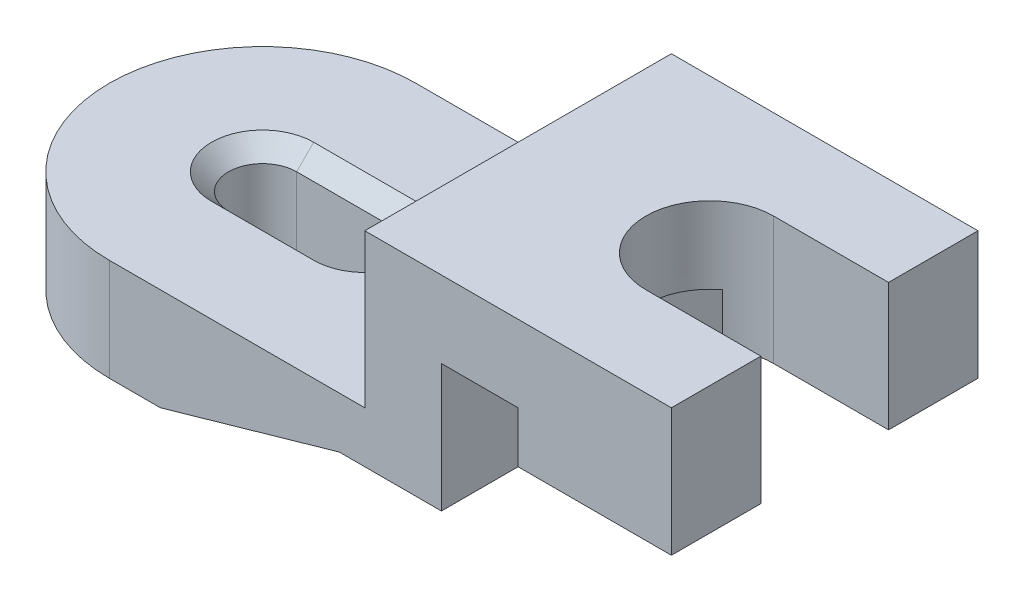
ISO-10303-21;
HEADER;
FILE_DESCRIPTION(('STEP AP214'),'2;1');
FILE_NAME('part.step','',(''),(''),'','','');
FILE_SCHEMA(('AUTOMOTIVE_DESIGN { 1 0 10303 214 1 1 1 1 }'));
ENDSEC;
DATA;
#1=APPLICATION_CONTEXT('core data for automotive mechanical design processes');
#2=APPLICATION_PROTOCOL_DEFINITION('international standard','automotive_design',2000,#1);
#3=PRODUCT_CONTEXT('',#1,'mechanical');
#4=PRODUCT('Part','Part','',(#3));
#5=PRODUCT_RELATED_PRODUCT_CATEGORY('part','',(#4));
#6=PRODUCT_DEFINITION_FORMATION('','',#4);
#7=PRODUCT_DEFINITION_CONTEXT('part definition',#1,'design');
#8=PRODUCT_DEFINITION('design','',#6,#7);
#9=PRODUCT_DEFINITION_SHAPE('','',#8);
#10=(LENGTH_UNIT() NAMED_UNIT(*) SI_UNIT(.MILLI.,.METRE.));
#11=(NAMED_UNIT(*) PLANE_ANGLE_UNIT() SI_UNIT($,.RADIAN.));
#12=(NAMED_UNIT(*) SI_UNIT($,.STERADIAN.) SOLID_ANGLE_UNIT());
#13=UNCERTAINTY_MEASURE_WITH_UNIT(LENGTH_MEASURE(1.E-05),#10,'distance_accuracy_value','');
#14=(GEOMETRIC_REPRESENTATION_CONTEXT(3) GLOBAL_UNCERTAINTY_ASSIGNED_CONTEXT((#13)) GLOBAL_UNIT_ASSIGNED_CONTEXT((#10,
#11,#12)) REPRESENTATION_CONTEXT('',''));
#15=CARTESIAN_POINT('',(0.,0.,0.));
#16=DIRECTION('',(0.,0.,1.));
#17=DIRECTION('',(1.,0.,0.));
#18=AXIS2_PLACEMENT_3D('',#15,#16,#17);
#19=CARTESIAN_POINT('',(0.,0.,0.));
#20=DIRECTION('',(0.,1.,0.));
#21=DIRECTION('',(0.,0.,1.));
#22=AXIS2_PLACEMENT_3D('',#19,#20,#21);
#23=PLANE('',#22);
#24=DIRECTION('',(0.,0.,-1.));
#25=VECTOR('',#24,1.);
#26=CARTESIAN_POINT('',(6.00000000000001,0.,208.));
#27=LINE('',#26,#25);
#28=CARTESIAN_POINT('',(6.00000000000001,0.,18.));
#29=VERTEX_POINT('',#28);
#30=CARTESIAN_POINT('',(6.00000000000001,0.,4.));
#31=VERTEX_POINT('',#30);
#32=EDGE_CURVE('E214',#29,#31,#27,.T.);
#33=ORIENTED_EDGE('',*,*,#32,.F.);
#34=DIRECTION('',(1.,0.,0.));
#35=VECTOR('',#34,1.);
#36=CARTESIAN_POINT('',(0.,0.,18.));
#37=LINE('',#36,#35);
#38=CARTESIAN_POINT('',(0.,0.,18.));
#39=VERTEX_POINT('',#38);
#40=EDGE_CURVE('E222',#39,#29,#37,.T.);
#41=ORIENTED_EDGE('',*,*,#40,.F.);
#42=CARTESIAN_POINT('',(0.,0.,0.));
#43=DIRECTION('',(0.,1.,0.));
#44=DIRECTION('',(0.,0.,1.));
#45=AXIS2_PLACEMENT_3D('',#42,#43,#44);
#46=CIRCLE('',#45,18.);
#47=CARTESIAN_POINT('',(0.,0.,-18.));
#48=VERTEX_POINT('',#47);
#49=EDGE_CURVE('E254',#48,#39,#46,.T.);
#50=ORIENTED_EDGE('',*,*,#49,.F.);
#51=DIRECTION('',(1.,0.,0.));
#52=VECTOR('',#51,1.);
#53=CARTESIAN_POINT('',(0.,0.,-18.));
#54=LINE('',#53,#52);
#55=CARTESIAN_POINT('',(6.00000000000001,0.,-18.));
#56=VERTEX_POINT('',#55);
#57=EDGE_CURVE('E234',#48,#56,#54,.T.);
#58=ORIENTED_EDGE('',*,*,#57,.T.);
#59=CARTESIAN_POINT('',(6.00000000000001,0.,-4.));
#60=VERTEX_POINT('',#59);
#61=EDGE_CURVE('E226',#60,#56,#27,.T.);
#62=ORIENTED_EDGE('',*,*,#61,.F.);
#63=DIRECTION('',(-1.,0.,0.));
#64=VECTOR('',#63,1.);
#65=CARTESIAN_POINT('',(0.,0.,-3.99999999999999));
#66=LINE('',#65,#64);
#67=CARTESIAN_POINT('',(0.,0.,-3.99999999999999));
#68=VERTEX_POINT('',#67);
#69=EDGE_CURVE('E259',#60,#68,#66,.T.);
#70=ORIENTED_EDGE('',*,*,#69,.T.);
#71=CARTESIAN_POINT('',(0.,0.,0.));
#72=DIRECTION('',(0.,1.,0.));
#73=DIRECTION('',(0.,0.,1.));
#74=AXIS2_PLACEMENT_3D('',#71,#72,#73);
#75=CIRCLE('',#74,3.99999999999999);
#76=CARTESIAN_POINT('',(0.,0.,3.99999999999999));
#77=VERTEX_POINT('',#76);
#78=EDGE_CURVE('E262',#68,#77,#75,.T.);
#79=ORIENTED_EDGE('',*,*,#78,.T.);
#80=DIRECTION('',(1.,0.,0.));
#81=VECTOR('',#80,1.);
#82=CARTESIAN_POINT('',(0.,0.,3.99999999999999));
#83=LINE('',#82,#81);
#84=EDGE_CURVE('E227',#77,#31,#83,.T.);
#85=ORIENTED_EDGE('',*,*,#84,.T.);
#86=EDGE_LOOP('',(#33,#41,#50,#58,#62,#70,#79,#85));
#87=FACE_BOUND('',#86,.T.);
#88=ADVANCED_FACE('F43',(#87),#23,.F.);
#89=CARTESIAN_POINT('',(0.,0.,-18.));
#90=DIRECTION('',(0.,0.,1.));
#91=DIRECTION('',(1.,0.,0.));
#92=AXIS2_PLACEMENT_3D('',#89,#90,#91);
#93=PLANE('',#92);
#94=DIRECTION('',(1.,0.,0.));
#95=VECTOR('',#94,1.);
#96=CARTESIAN_POINT('',(0.,5.99999999999999,-18.));
#97=LINE('',#96,#95);
#98=CARTESIAN_POINT('',(27.,6.,-18.));
#99=VERTEX_POINT('',#98);
#100=CARTESIAN_POINT('',(39.,6.,-18.));
#101=VERTEX_POINT('',#100);
#102=EDGE_CURVE('E59',#99,#101,#97,.T.);
#103=ORIENTED_EDGE('',*,*,#102,.F.);
#104=DIRECTION('',(0.961523947640823,0.274721127897378,0.));
#105=VECTOR('',#104,1.);
#106=CARTESIAN_POINT('',(0.452830188679243,-1.58490566037736,-18.));
#107=LINE('',#106,#105);
#108=EDGE_CURVE('E219',#56,#99,#107,.T.);
#109=ORIENTED_EDGE('',*,*,#108,.F.);
#110=ORIENTED_EDGE('',*,*,#57,.F.);
#111=DIRECTION('',(0.,1.,0.));
#112=VECTOR('',#111,1.);
#113=CARTESIAN_POINT('',(0.,0.,-18.));
#114=LINE('',#113,#112);
#115=CARTESIAN_POINT('',(0.,12.,-18.));
#116=VERTEX_POINT('',#115);
#117=EDGE_CURVE('E249',#48,#116,#114,.T.);
#118=ORIENTED_EDGE('',*,*,#117,.T.);
#119=DIRECTION('',(1.,0.,0.));
#120=VECTOR('',#119,1.);
#121=CARTESIAN_POINT('',(0.,12.,-18.));
#122=LINE('',#121,#120);
#123=CARTESIAN_POINT('',(30.,12.,-18.));
#124=VERTEX_POINT('',#123);
#125=EDGE_CURVE('E232',#116,#124,#122,.T.);
#126=ORIENTED_EDGE('',*,*,#125,.T.);
#127=DIRECTION('',(0.,-1.,0.));
#128=VECTOR('',#127,1.);
#129=CARTESIAN_POINT('',(30.,12.,-18.));
#130=LINE('',#129,#128);
#131=CARTESIAN_POINT('',(30.,30.,-18.));
#132=VERTEX_POINT('',#131);
#133=EDGE_CURVE('E330',#132,#124,#130,.T.);
#134=ORIENTED_EDGE('',*,*,#133,.F.);
#135=DIRECTION('',(-1.,0.,0.));
#136=VECTOR('',#135,1.);
#137=CARTESIAN_POINT('',(30.,30.,-18.));
#138=LINE('',#137,#136);
#139=CARTESIAN_POINT('',(66.,30.,-18.));
#140=VERTEX_POINT('',#139);
#141=EDGE_CURVE('E335',#140,#132,#138,.T.);
#142=ORIENTED_EDGE('',*,*,#141,.F.);
#143=DIRECTION('',(0.,1.,0.));
#144=VECTOR('',#143,1.);
#145=CARTESIAN_POINT('',(66.,0.,-18.));
#146=LINE('',#145,#144);
#147=CARTESIAN_POINT('',(66.,15.,-18.));
#148=VERTEX_POINT('',#147);
#149=EDGE_CURVE('E326',#148,#140,#146,.T.);
#150=ORIENTED_EDGE('',*,*,#149,.F.);
#151=DIRECTION('',(-1.,0.,0.));
#152=VECTOR('',#151,1.);
#153=CARTESIAN_POINT('',(0.,15.,-18.));
#154=LINE('',#153,#152);
#155=CARTESIAN_POINT('',(48.,15.,-18.));
#156=VERTEX_POINT('',#155);
#157=EDGE_CURVE('E432',#148,#156,#154,.T.);
#158=ORIENTED_EDGE('',*,*,#157,.T.);
#159=DIRECTION('',(0.,-1.,0.));
#160=VECTOR('',#159,1.);
#161=CARTESIAN_POINT('',(48.,0.,-18.));
#162=LINE('',#161,#160);
#163=CARTESIAN_POINT('',(48.,21.,-18.));
#164=VERTEX_POINT('',#163);
#165=EDGE_CURVE('E297',#164,#156,#162,.T.);
#166=ORIENTED_EDGE('',*,*,#165,.F.);
#167=DIRECTION('',(-1.,0.,0.));
#168=VECTOR('',#167,1.);
#169=CARTESIAN_POINT('',(0.,21.,-18.));
#170=LINE('',#169,#168);
#171=CARTESIAN_POINT('',(39.,21.,-18.));
#172=VERTEX_POINT('',#171);
#173=EDGE_CURVE('E311',#164,#172,#170,.T.);
#174=ORIENTED_EDGE('',*,*,#173,.T.);
#175=DIRECTION('',(0.,-1.,0.));
#176=VECTOR('',#175,1.);
#177=CARTESIAN_POINT('',(39.,0.,-18.));
#178=LINE('',#177,#176);
#179=EDGE_CURVE('E291',#172,#101,#178,.T.);
#180=ORIENTED_EDGE('',*,*,#179,.T.);
#181=EDGE_LOOP('',(#103,#109,#110,#118,#126,#134,#142,#150,#158,#166,#174,#180));
#182=FACE_BOUND('',#181,.T.);
#183=ADVANCED_FACE('F443',(#182),#93,.F.);
#184=CARTESIAN_POINT('',(0.,0.,18.));
#185=DIRECTION('',(0.,0.,1.));
#186=DIRECTION('',(1.,0.,0.));
#187=AXIS2_PLACEMENT_3D('',#184,#185,#186);
#188=PLANE('',#187);
#189=DIRECTION('',(0.961523947640823,0.274721127897378,0.));
#190=VECTOR('',#189,1.);
#191=CARTESIAN_POINT('',(0.452830188679243,-1.58490566037736,18.));
#192=LINE('',#191,#190);
#193=CARTESIAN_POINT('',(27.,6.,18.));
#194=VERTEX_POINT('',#193);
#195=EDGE_CURVE('E208',#29,#194,#192,.T.);
#196=ORIENTED_EDGE('',*,*,#195,.T.);
#197=DIRECTION('',(1.,0.,0.));
#198=VECTOR('',#197,1.);
#199=CARTESIAN_POINT('',(0.,5.99999999999999,18.));
#200=LINE('',#199,#198);
#201=CARTESIAN_POINT('',(39.,6.,18.));
#202=VERTEX_POINT('',#201);
#203=EDGE_CURVE('E283',#194,#202,#200,.T.);
#204=ORIENTED_EDGE('',*,*,#203,.T.);
#205=DIRECTION('',(0.,-1.,0.));
#206=VECTOR('',#205,1.);
#207=CARTESIAN_POINT('',(39.,0.,18.));
#208=LINE('',#207,#206);
#209=CARTESIAN_POINT('',(39.,21.,18.));
#210=VERTEX_POINT('',#209);
#211=EDGE_CURVE('E279',#210,#202,#208,.T.);
#212=ORIENTED_EDGE('',*,*,#211,.F.);
#213=DIRECTION('',(-1.,0.,0.));
#214=VECTOR('',#213,1.);
#215=CARTESIAN_POINT('',(0.,21.,18.));
#216=LINE('',#215,#214);
#217=CARTESIAN_POINT('',(48.,21.,18.));
#218=VERTEX_POINT('',#217);
#219=EDGE_CURVE('E307',#218,#210,#216,.T.);
#220=ORIENTED_EDGE('',*,*,#219,.F.);
#221=DIRECTION('',(0.,-1.,0.));
#222=VECTOR('',#221,1.);
#223=CARTESIAN_POINT('',(48.,0.,18.));
#224=LINE('',#223,#222);
#225=CARTESIAN_POINT('',(48.,15.,18.));
#226=VERTEX_POINT('',#225);
#227=EDGE_CURVE('E298',#218,#226,#224,.T.);
#228=ORIENTED_EDGE('',*,*,#227,.T.);
#229=DIRECTION('',(-1.,0.,0.));
#230=VECTOR('',#229,1.);
#231=CARTESIAN_POINT('',(0.,15.,18.));
#232=LINE('',#231,#230);
#233=CARTESIAN_POINT('',(66.,15.,18.));
#234=VERTEX_POINT('',#233);
#235=EDGE_CURVE('E433',#234,#226,#232,.T.);
#236=ORIENTED_EDGE('',*,*,#235,.F.);
#237=DIRECTION('',(0.,1.,0.));
#238=VECTOR('',#237,1.);
#239=CARTESIAN_POINT('',(66.,30.,18.));
#240=LINE('',#239,#238);
#241=CARTESIAN_POINT('',(66.,30.,18.));
#242=VERTEX_POINT('',#241);
#243=EDGE_CURVE('E323',#234,#242,#240,.T.);
#244=ORIENTED_EDGE('',*,*,#243,.T.);
#245=DIRECTION('',(-1.,0.,0.));
#246=VECTOR('',#245,1.);
#247=CARTESIAN_POINT('',(30.,30.,18.));
#248=LINE('',#247,#246);
#249=CARTESIAN_POINT('',(30.,30.,18.));
#250=VERTEX_POINT('',#249);
#251=EDGE_CURVE('E336',#242,#250,#248,.T.);
#252=ORIENTED_EDGE('',*,*,#251,.T.);
#253=DIRECTION('',(0.,-1.,0.));
#254=VECTOR('',#253,1.);
#255=CARTESIAN_POINT('',(30.,12.,18.));
#256=LINE('',#255,#254);
#257=CARTESIAN_POINT('',(30.,12.,18.));
#258=VERTEX_POINT('',#257);
#259=EDGE_CURVE('E334',#250,#258,#256,.T.);
#260=ORIENTED_EDGE('',*,*,#259,.T.);
#261=DIRECTION('',(1.,0.,0.));
#262=VECTOR('',#261,1.);
#263=CARTESIAN_POINT('',(0.,12.,18.));
#264=LINE('',#263,#262);
#265=CARTESIAN_POINT('',(0.,12.,18.));
#266=VERTEX_POINT('',#265);
#267=EDGE_CURVE('E244',#266,#258,#264,.T.);
#268=ORIENTED_EDGE('',*,*,#267,.F.);
#269=DIRECTION('',(0.,1.,0.));
#270=VECTOR('',#269,1.);
#271=CARTESIAN_POINT('',(0.,0.,18.));
#272=LINE('',#271,#270);
#273=EDGE_CURVE('E231',#39,#266,#272,.T.);
#274=ORIENTED_EDGE('',*,*,#273,.F.);
#275=ORIENTED_EDGE('',*,*,#40,.T.);
#276=EDGE_LOOP('',(#196,#204,#212,#220,#228,#236,#244,#252,#260,#268,#274,#275));
#277=FACE_BOUND('',#276,.T.);
#278=ADVANCED_FACE('F233',(#277),#188,.T.);
#279=CARTESIAN_POINT('',(0.,-8.,3.99999999999999));
#280=DIRECTION('',(0.,0.,1.));
#281=DIRECTION('',(1.,0.,0.));
#282=AXIS2_PLACEMENT_3D('',#279,#280,#281);
#283=PLANE('',#282);
#284=DIRECTION('',(0.961523947640823,0.274721127897378,0.));
#285=VECTOR('',#284,1.);
#286=CARTESIAN_POINT('',(-1.66037735849057,-2.18867924528302,3.99999999999999));
#287=LINE('',#286,#285);
#288=CARTESIAN_POINT('',(12.,1.71428571428571,3.99999999999999));
#289=VERTEX_POINT('',#288);
#290=EDGE_CURVE('E216',#31,#289,#287,.T.);
#291=ORIENTED_EDGE('',*,*,#290,.F.);
#292=ORIENTED_EDGE('',*,*,#84,.F.);
#293=DIRECTION('',(0.,1.,0.));
#294=VECTOR('',#293,1.);
#295=CARTESIAN_POINT('',(0.,-8.,3.99999999999999));
#296=LINE('',#295,#294);
#297=CARTESIAN_POINT('',(0.,10.,3.99999999999999));
#298=VERTEX_POINT('',#297);
#299=EDGE_CURVE('E349',#77,#298,#296,.T.);
#300=ORIENTED_EDGE('',*,*,#299,.T.);
#301=DIRECTION('',(1.,0.,0.));
#302=VECTOR('',#301,1.);
#303=CARTESIAN_POINT('',(0.,10.,3.99999999999999));
#304=LINE('',#303,#302);
#305=CARTESIAN_POINT('',(12.,10.,3.99999999999999));
#306=VERTEX_POINT('',#305);
#307=EDGE_CURVE('E245',#298,#306,#304,.T.);
#308=ORIENTED_EDGE('',*,*,#307,.T.);
#309=DIRECTION('',(0.,1.,0.));
#310=VECTOR('',#309,1.);
#311=CARTESIAN_POINT('',(12.,-8.,3.99999999999999));
#312=LINE('',#311,#310);
#313=EDGE_CURVE('E343',#289,#306,#312,.T.);
#314=ORIENTED_EDGE('',*,*,#313,.F.);
#315=EDGE_LOOP('',(#291,#292,#300,#308,#314));
#316=FACE_BOUND('',#315,.T.);
#317=ADVANCED_FACE('F392',(#316),#283,.F.);
#318=CARTESIAN_POINT('',(0.,-8.,-3.99999999999999));
#319=DIRECTION('',(0.,0.,-1.));
#320=DIRECTION('',(-1.,0.,0.));
#321=AXIS2_PLACEMENT_3D('',#318,#319,#320);
#322=PLANE('',#321);
#323=DIRECTION('',(-0.961523947640823,-0.274721127897378,0.));
#324=VECTOR('',#323,1.);
#325=CARTESIAN_POINT('',(-1.66037735849057,-2.18867924528302,-3.99999999999999));
#326=LINE('',#325,#324);
#327=CARTESIAN_POINT('',(12.,1.71428571428571,-3.99999999999999));
#328=VERTEX_POINT('',#327);
#329=EDGE_CURVE('E408',#328,#60,#326,.T.);
#330=ORIENTED_EDGE('',*,*,#329,.F.);
#331=DIRECTION('',(0.,1.,0.));
#332=VECTOR('',#331,1.);
#333=CARTESIAN_POINT('',(12.,-8.,-3.99999999999999));
#334=LINE('',#333,#332);
#335=CARTESIAN_POINT('',(12.,10.,-3.99999999999999));
#336=VERTEX_POINT('',#335);
#337=EDGE_CURVE('E353',#328,#336,#334,.T.);
#338=ORIENTED_EDGE('',*,*,#337,.T.);
#339=DIRECTION('',(-1.,0.,0.));
#340=VECTOR('',#339,1.);
#341=CARTESIAN_POINT('',(0.,10.,-3.99999999999999));
#342=LINE('',#341,#340);
#343=CARTESIAN_POINT('',(0.,10.,-3.99999999999999));
#344=VERTEX_POINT('',#343);
#345=EDGE_CURVE('E372',#336,#344,#342,.T.);
#346=ORIENTED_EDGE('',*,*,#345,.T.);
#347=DIRECTION('',(0.,1.,0.));
#348=VECTOR('',#347,1.);
#349=CARTESIAN_POINT('',(0.,-8.,-3.99999999999999));
#350=LINE('',#349,#348);
#351=EDGE_CURVE('E351',#68,#344,#350,.T.);
#352=ORIENTED_EDGE('',*,*,#351,.F.);
#353=ORIENTED_EDGE('',*,*,#69,.F.);
#354=EDGE_LOOP('',(#330,#338,#346,#352,#353));
#355=FACE_BOUND('',#354,.T.);
#356=ADVANCED_FACE('F409',(#355),#322,.F.);
#357=CARTESIAN_POINT('',(12.,-8.,0.));
#358=DIRECTION('',(0.,1.,0.));
#359=DIRECTION('',(0.,0.,1.));
#360=AXIS2_PLACEMENT_3D('',#357,#358,#359);
#361=CYLINDRICAL_SURFACE('',#360,3.99999999999999);
#362=CARTESIAN_POINT('',(12.,1.71428571428571,0.));
#363=DIRECTION('',(0.274721127897378,-0.961523947640823,0.));
#364=DIRECTION('',(0.961523947640823,0.274721127897378,0.));
#365=AXIS2_PLACEMENT_3D('',#362,#363,#364);
#366=ELLIPSE('',#365,4.16006279387457,3.99999999999999);
#367=EDGE_CURVE('E11',#289,#328,#366,.F.);
#368=ORIENTED_EDGE('',*,*,#367,.F.);
#369=ORIENTED_EDGE('',*,*,#313,.T.);
#370=CARTESIAN_POINT('',(12.,10.,0.));
#371=DIRECTION('',(0.,1.,0.));
#372=DIRECTION('',(0.,0.,1.));
#373=AXIS2_PLACEMENT_3D('',#370,#371,#372);
#374=CIRCLE('',#373,3.99999999999999);
#375=EDGE_CURVE('E379',#306,#336,#374,.T.);
#376=ORIENTED_EDGE('',*,*,#375,.T.);
#377=ORIENTED_EDGE('',*,*,#337,.F.);
#378=EDGE_LOOP('',(#368,#369,#376,#377));
#379=FACE_BOUND('',#378,.T.);
#380=ADVANCED_FACE('F415',(#379),#361,.F.);
#381=CARTESIAN_POINT('',(39.,0.,78.));
#382=DIRECTION('',(-1.,0.,0.));
#383=DIRECTION('',(0.,0.,1.));
#384=AXIS2_PLACEMENT_3D('',#381,#382,#383);
#385=PLANE('',#384);
#386=DIRECTION('',(0.,0.,1.));
#387=VECTOR('',#386,1.);
#388=CARTESIAN_POINT('',(39.,6.,78.));
#389=LINE('',#388,#387);
#390=EDGE_CURVE('E51',#101,#202,#389,.T.);
#391=ORIENTED_EDGE('',*,*,#390,.F.);
#392=ORIENTED_EDGE('',*,*,#179,.F.);
#393=DIRECTION('',(0.,0.,-1.));
#394=VECTOR('',#393,1.);
#395=CARTESIAN_POINT('',(39.,21.,78.));
#396=LINE('',#395,#394);
#397=EDGE_CURVE('E292',#210,#172,#396,.T.);
#398=ORIENTED_EDGE('',*,*,#397,.F.);
#399=ORIENTED_EDGE('',*,*,#211,.T.);
#400=EDGE_LOOP('',(#391,#392,#398,#399));
#401=FACE_BOUND('',#400,.T.);
#402=ADVANCED_FACE('F287',(#401),#385,.F.);
#403=CARTESIAN_POINT('',(52.5,-60.,0.));
#404=DIRECTION('',(0.,1.,0.));
#405=DIRECTION('',(0.,0.,1.));
#406=AXIS2_PLACEMENT_3D('',#403,#404,#405);
#407=CYLINDRICAL_SURFACE('',#406,7.5);
#408=DIRECTION('',(0.,1.,0.));
#409=VECTOR('',#408,1.);
#410=CARTESIAN_POINT('',(52.5,-60.,7.5));
#411=LINE('',#410,#409);
#412=CARTESIAN_POINT('',(52.5,15.,7.5));
#413=VERTEX_POINT('',#412);
#414=CARTESIAN_POINT('',(52.5,30.,7.5));
#415=VERTEX_POINT('',#414);
#416=EDGE_CURVE('E325',#413,#415,#411,.T.);
#417=ORIENTED_EDGE('',*,*,#416,.F.);
#418=CARTESIAN_POINT('',(52.5,15.,0.));
#419=DIRECTION('',(0.,1.,0.));
#420=DIRECTION('',(0.,0.,1.));
#421=AXIS2_PLACEMENT_3D('',#418,#419,#420);
#422=CIRCLE('',#421,7.5);
#423=CARTESIAN_POINT('',(48.,15.,5.99999999999999));
#424=VERTEX_POINT('',#423);
#425=EDGE_CURVE('E426',#413,#424,#422,.F.);
#426=ORIENTED_EDGE('',*,*,#425,.T.);
#427=DIRECTION('',(0.,1.,0.));
#428=VECTOR('',#427,1.);
#429=CARTESIAN_POINT('',(48.,-60.,5.99999999999999));
#430=LINE('',#429,#428);
#431=CARTESIAN_POINT('',(48.,21.,5.99999999999999));
#432=VERTEX_POINT('',#431);
#433=EDGE_CURVE('E273',#432,#424,#430,.F.);
#434=ORIENTED_EDGE('',*,*,#433,.F.);
#435=CARTESIAN_POINT('',(52.5,21.,0.));
#436=DIRECTION('',(0.,1.,0.));
#437=DIRECTION('',(0.,0.,1.));
#438=AXIS2_PLACEMENT_3D('',#435,#436,#437);
#439=CIRCLE('',#438,7.5);
#440=CARTESIAN_POINT('',(48.,21.,-6.00000000000001));
#441=VERTEX_POINT('',#440);
#442=EDGE_CURVE('E275',#432,#441,#439,.F.);
#443=ORIENTED_EDGE('',*,*,#442,.T.);
#444=DIRECTION('',(0.,1.,0.));
#445=VECTOR('',#444,1.);
#446=CARTESIAN_POINT('',(48.,-60.,-6.));
#447=LINE('',#446,#445);
#448=CARTESIAN_POINT('',(48.,15.,-6.));
#449=VERTEX_POINT('',#448);
#450=EDGE_CURVE('E267',#449,#441,#447,.T.);
#451=ORIENTED_EDGE('',*,*,#450,.F.);
#452=CARTESIAN_POINT('',(52.5,15.,-7.5));
#453=VERTEX_POINT('',#452);
#454=EDGE_CURVE('E67',#449,#453,#422,.F.);
#455=ORIENTED_EDGE('',*,*,#454,.T.);
#456=DIRECTION('',(0.,1.,0.));
#457=VECTOR('',#456,1.);
#458=CARTESIAN_POINT('',(52.5,-60.,-7.5));
#459=LINE('',#458,#457);
#460=CARTESIAN_POINT('',(52.5,30.,-7.5));
#461=VERTEX_POINT('',#460);
#462=EDGE_CURVE('E324',#453,#461,#459,.T.);
#463=ORIENTED_EDGE('',*,*,#462,.T.);
#464=CARTESIAN_POINT('',(52.5,30.,0.));
#465=DIRECTION('',(0.,1.,0.));
#466=DIRECTION('',(0.,0.,1.));
#467=AXIS2_PLACEMENT_3D('',#464,#465,#466);
#468=CIRCLE('',#467,7.5);
#469=EDGE_CURVE('E313',#461,#415,#468,.T.);
#470=ORIENTED_EDGE('',*,*,#469,.T.);
#471=EDGE_LOOP('',(#417,#426,#434,#443,#451,#455,#463,#470));
#472=FACE_BOUND('',#471,.T.);
#473=ADVANCED_FACE('F503',(#472),#407,.F.);
#474=CARTESIAN_POINT('',(30.,30.,-18.));
#475=DIRECTION('',(0.,1.,0.));
#476=DIRECTION('',(0.,0.,1.));
#477=AXIS2_PLACEMENT_3D('',#474,#475,#476);
#478=PLANE('',#477);
#479=ORIENTED_EDGE('',*,*,#469,.F.);
#480=DIRECTION('',(1.,0.,0.));
#481=VECTOR('',#480,1.);
#482=CARTESIAN_POINT('',(0.,30.,-7.5));
#483=LINE('',#482,#481);
#484=CARTESIAN_POINT('',(66.,30.,-7.5));
#485=VERTEX_POINT('',#484);
#486=EDGE_CURVE('E316',#461,#485,#483,.T.);
#487=ORIENTED_EDGE('',*,*,#486,.T.);
#488=DIRECTION('',(0.,0.,1.));
#489=VECTOR('',#488,1.);
#490=CARTESIAN_POINT('',(66.,30.,-18.));
#491=LINE('',#490,#489);
#492=EDGE_CURVE('E347',#140,#485,#491,.T.);
#493=ORIENTED_EDGE('',*,*,#492,.F.);
#494=ORIENTED_EDGE('',*,*,#141,.T.);
#495=DIRECTION('',(0.,0.,1.));
#496=VECTOR('',#495,1.);
#497=CARTESIAN_POINT('',(30.,30.,-18.));
#498=LINE('',#497,#496);
#499=EDGE_CURVE('E344',#132,#250,#498,.T.);
#500=ORIENTED_EDGE('',*,*,#499,.T.);
#501=ORIENTED_EDGE('',*,*,#251,.F.);
#502=CARTESIAN_POINT('',(66.,30.,7.49999999999999));
#503=VERTEX_POINT('',#502);
#504=EDGE_CURVE('E337',#503,#242,#491,.T.);
#505=ORIENTED_EDGE('',*,*,#504,.F.);
#506=DIRECTION('',(1.,0.,0.));
#507=VECTOR('',#506,1.);
#508=CARTESIAN_POINT('',(0.,30.,7.5));
#509=LINE('',#508,#507);
#510=EDGE_CURVE('E320',#415,#503,#509,.T.);
#511=ORIENTED_EDGE('',*,*,#510,.F.);
#512=EDGE_LOOP('',(#479,#487,#493,#494,#500,#501,#505,#511));
#513=FACE_BOUND('',#512,.T.);
#514=ADVANCED_FACE('F501',(#513),#478,.T.);
#515=CARTESIAN_POINT('',(66.,30.,-18.));
#516=DIRECTION('',(1.,0.,0.));
#517=DIRECTION('',(0.,0.,-1.));
#518=AXIS2_PLACEMENT_3D('',#515,#516,#517);
#519=PLANE('',#518);
#520=DIRECTION('',(0.,0.,-1.));
#521=VECTOR('',#520,1.);
#522=CARTESIAN_POINT('',(66.,15.,91.));
#523=LINE('',#522,#521);
#524=CARTESIAN_POINT('',(66.,15.,-7.50000000000001));
#525=VERTEX_POINT('',#524);
#526=EDGE_CURVE('E418',#525,#148,#523,.T.);
#527=ORIENTED_EDGE('',*,*,#526,.T.);
#528=ORIENTED_EDGE('',*,*,#149,.T.);
#529=ORIENTED_EDGE('',*,*,#492,.T.);
#530=DIRECTION('',(0.,-1.,0.));
#531=VECTOR('',#530,1.);
#532=CARTESIAN_POINT('',(66.,30.,-7.5));
#533=LINE('',#532,#531);
#534=EDGE_CURVE('E266',#485,#525,#533,.T.);
#535=ORIENTED_EDGE('',*,*,#534,.T.);
#536=EDGE_LOOP('',(#527,#528,#529,#535));
#537=FACE_BOUND('',#536,.T.);
#538=ADVANCED_FACE('F499',(#537),#519,.T.);
#539=CARTESIAN_POINT('',(0.,12.,0.));
#540=DIRECTION('',(0.,-1.,0.));
#541=DIRECTION('',(0.,0.,-1.));
#542=AXIS2_PLACEMENT_3D('',#539,#540,#541);
#543=CYLINDRICAL_SURFACE('',#542,18.);
#544=CARTESIAN_POINT('',(0.,12.,0.));
#545=DIRECTION('',(0.,1.,0.));
#546=DIRECTION('',(0.,0.,1.));
#547=AXIS2_PLACEMENT_3D('',#544,#545,#546);
#548=CIRCLE('',#547,18.);
#549=EDGE_CURVE('E253',#116,#266,#548,.T.);
#550=ORIENTED_EDGE('',*,*,#549,.F.);
#551=ORIENTED_EDGE('',*,*,#117,.F.);
#552=ORIENTED_EDGE('',*,*,#49,.T.);
#553=ORIENTED_EDGE('',*,*,#273,.T.);
#554=EDGE_LOOP('',(#550,#551,#552,#553));
#555=FACE_BOUND('',#554,.T.);
#556=ADVANCED_FACE('F44',(#555),#543,.T.);
#557=CARTESIAN_POINT('',(0.,12.,0.));
#558=DIRECTION('',(0.,1.,0.));
#559=DIRECTION('',(0.,0.,1.));
#560=AXIS2_PLACEMENT_3D('',#557,#558,#559);
#561=PLANE('',#560);
#562=CARTESIAN_POINT('',(0.,12.,0.));
#563=DIRECTION('',(0.,1.,0.));
#564=DIRECTION('',(0.,0.,1.));
#565=AXIS2_PLACEMENT_3D('',#562,#563,#564);
#566=CIRCLE('',#565,6.);
#567=CARTESIAN_POINT('',(0.,12.,-6.));
#568=VERTEX_POINT('',#567);
#569=CARTESIAN_POINT('',(0.,12.,6.));
#570=VERTEX_POINT('',#569);
#571=EDGE_CURVE('E354',#568,#570,#566,.T.);
#572=ORIENTED_EDGE('',*,*,#571,.F.);
#573=DIRECTION('',(-1.,0.,0.));
#574=VECTOR('',#573,1.);
#575=CARTESIAN_POINT('',(0.,12.,-6.));
#576=LINE('',#575,#574);
#577=CARTESIAN_POINT('',(12.,12.,-6.));
#578=VERTEX_POINT('',#577);
#579=EDGE_CURVE('E364',#578,#568,#576,.T.);
#580=ORIENTED_EDGE('',*,*,#579,.F.);
#581=CARTESIAN_POINT('',(12.,12.,0.));
#582=DIRECTION('',(0.,1.,0.));
#583=DIRECTION('',(0.,0.,1.));
#584=AXIS2_PLACEMENT_3D('',#581,#582,#583);
#585=CIRCLE('',#584,6.);
#586=CARTESIAN_POINT('',(12.,12.,6.));
#587=VERTEX_POINT('',#586);
#588=EDGE_CURVE('E363',#587,#578,#585,.T.);
#589=ORIENTED_EDGE('',*,*,#588,.F.);
#590=DIRECTION('',(1.,0.,0.));
#591=VECTOR('',#590,1.);
#592=CARTESIAN_POINT('',(0.,12.,6.));
#593=LINE('',#592,#591);
#594=EDGE_CURVE('E356',#570,#587,#593,.T.);
#595=ORIENTED_EDGE('',*,*,#594,.F.);
#596=EDGE_LOOP('',(#572,#580,#589,#595));
#597=FACE_BOUND('',#596,.T.);
#598=ORIENTED_EDGE('',*,*,#549,.T.);
#599=ORIENTED_EDGE('',*,*,#267,.T.);
#600=DIRECTION('',(0.,0.,1.));
#601=VECTOR('',#600,1.);
#602=CARTESIAN_POINT('',(30.,12.,0.));
#603=LINE('',#602,#601);
#604=EDGE_CURVE('E237',#124,#258,#603,.T.);
#605=ORIENTED_EDGE('',*,*,#604,.F.);
#606=ORIENTED_EDGE('',*,*,#125,.F.);
#607=EDGE_LOOP('',(#598,#599,#605,#606));
#608=FACE_BOUND('',#607,.T.);
#609=ADVANCED_FACE('F469',(#597,#608),#561,.T.);
#610=CARTESIAN_POINT('',(0.,12.,0.));
#611=DIRECTION('',(0.,1.,0.));
#612=DIRECTION('',(0.,0.,1.));
#613=AXIS2_PLACEMENT_3D('',#610,#611,#612);
#614=CONICAL_SURFACE('',#613,6.,0.78539816339745);
#615=ORIENTED_EDGE('',*,*,#571,.T.);
#616=DIRECTION('',(0.,0.707106781186546,0.707106781186549));
#617=VECTOR('',#616,1.);
#618=CARTESIAN_POINT('',(0.,12.,6.));
#619=LINE('',#618,#617);
#620=EDGE_CURVE('E369',#298,#570,#619,.T.);
#621=ORIENTED_EDGE('',*,*,#620,.F.);
#622=CARTESIAN_POINT('',(0.,10.,0.));
#623=DIRECTION('',(0.,1.,0.));
#624=DIRECTION('',(0.,0.,1.));
#625=AXIS2_PLACEMENT_3D('',#622,#623,#624);
#626=CIRCLE('',#625,3.99999999999999);
#627=EDGE_CURVE('E370',#344,#298,#626,.T.);
#628=ORIENTED_EDGE('',*,*,#627,.F.);
#629=DIRECTION('',(0.,0.707106781186546,-0.707106781186549));
#630=VECTOR('',#629,1.);
#631=CARTESIAN_POINT('',(0.,12.,-6.));
#632=LINE('',#631,#630);
#633=EDGE_CURVE('E250',#344,#568,#632,.T.);
#634=ORIENTED_EDGE('',*,*,#633,.T.);
#635=EDGE_LOOP('',(#615,#621,#628,#634));
#636=FACE_BOUND('',#635,.T.);
#637=ADVANCED_FACE('F475',(#636),#614,.F.);
#638=CARTESIAN_POINT('',(0.,12.,-6.));
#639=DIRECTION('',(0.,-0.707106781186549,-0.707106781186546));
#640=DIRECTION('',(0.,0.707106781186546,-0.707106781186549));
#641=AXIS2_PLACEMENT_3D('',#638,#639,#640);
#642=PLANE('',#641);
#643=ORIENTED_EDGE('',*,*,#579,.T.);
#644=ORIENTED_EDGE('',*,*,#633,.F.);
#645=ORIENTED_EDGE('',*,*,#345,.F.);
#646=DIRECTION('',(0.,0.707106781186546,-0.707106781186549));
#647=VECTOR('',#646,1.);
#648=CARTESIAN_POINT('',(12.,12.,-6.));
#649=LINE('',#648,#647);
#650=EDGE_CURVE('E367',#336,#578,#649,.T.);
#651=ORIENTED_EDGE('',*,*,#650,.T.);
#652=EDGE_LOOP('',(#643,#644,#645,#651));
#653=FACE_BOUND('',#652,.T.);
#654=ADVANCED_FACE('F401',(#653),#642,.F.);
#655=CARTESIAN_POINT('',(12.,12.,0.));
#656=DIRECTION('',(0.,1.,0.));
#657=DIRECTION('',(0.,0.,1.));
#658=AXIS2_PLACEMENT_3D('',#655,#656,#657);
#659=CONICAL_SURFACE('',#658,6.,0.78539816339745);
#660=ORIENTED_EDGE('',*,*,#588,.T.);
#661=ORIENTED_EDGE('',*,*,#650,.F.);
#662=ORIENTED_EDGE('',*,*,#375,.F.);
#663=DIRECTION('',(0.,0.707106781186546,0.707106781186549));
#664=VECTOR('',#663,1.);
#665=CARTESIAN_POINT('',(12.,12.,6.));
#666=LINE('',#665,#664);
#667=EDGE_CURVE('E373',#306,#587,#666,.T.);
#668=ORIENTED_EDGE('',*,*,#667,.T.);
#669=EDGE_LOOP('',(#660,#661,#662,#668));
#670=FACE_BOUND('',#669,.T.);
#671=ADVANCED_FACE('F400',(#670),#659,.F.);
#672=CARTESIAN_POINT('',(0.,12.,6.));
#673=DIRECTION('',(0.,-0.707106781186549,0.707106781186546));
#674=DIRECTION('',(0.,-0.707106781186546,-0.707106781186549));
#675=AXIS2_PLACEMENT_3D('',#672,#673,#674);
#676=PLANE('',#675);
#677=ORIENTED_EDGE('',*,*,#594,.T.);
#678=ORIENTED_EDGE('',*,*,#667,.F.);
#679=ORIENTED_EDGE('',*,*,#307,.F.);
#680=ORIENTED_EDGE('',*,*,#620,.T.);
#681=EDGE_LOOP('',(#677,#678,#679,#680));
#682=FACE_BOUND('',#681,.T.);
#683=ADVANCED_FACE('F394',(#682),#676,.F.);
#684=CARTESIAN_POINT('',(0.,-8.,0.));
#685=DIRECTION('',(0.,1.,0.));
#686=DIRECTION('',(0.,0.,1.));
#687=AXIS2_PLACEMENT_3D('',#684,#685,#686);
#688=CYLINDRICAL_SURFACE('',#687,3.99999999999999);
#689=ORIENTED_EDGE('',*,*,#351,.T.);
#690=ORIENTED_EDGE('',*,*,#627,.T.);
#691=ORIENTED_EDGE('',*,*,#299,.F.);
#692=ORIENTED_EDGE('',*,*,#78,.F.);
#693=EDGE_LOOP('',(#689,#690,#691,#692));
#694=FACE_BOUND('',#693,.T.);
#695=ADVANCED_FACE('F481',(#694),#688,.F.);
#696=CARTESIAN_POINT('',(30.,12.,-18.));
#697=DIRECTION('',(-1.,0.,0.));
#698=DIRECTION('',(0.,0.,1.));
#699=AXIS2_PLACEMENT_3D('',#696,#697,#698);
#700=PLANE('',#699);
#701=ORIENTED_EDGE('',*,*,#133,.T.);
#702=ORIENTED_EDGE('',*,*,#604,.T.);
#703=ORIENTED_EDGE('',*,*,#259,.F.);
#704=ORIENTED_EDGE('',*,*,#499,.F.);
#705=EDGE_LOOP('',(#701,#702,#703,#704));
#706=FACE_BOUND('',#705,.T.);
#707=ADVANCED_FACE('F494',(#706),#700,.T.);
#708=CARTESIAN_POINT('',(66.,15.,7.49999999999999));
#709=VERTEX_POINT('',#708);
#710=EDGE_CURVE('E422',#234,#709,#523,.T.);
#711=ORIENTED_EDGE('',*,*,#710,.T.);
#712=DIRECTION('',(0.,-1.,0.));
#713=VECTOR('',#712,1.);
#714=CARTESIAN_POINT('',(66.,30.,7.5));
#715=LINE('',#714,#713);
#716=EDGE_CURVE('E264',#503,#709,#715,.T.);
#717=ORIENTED_EDGE('',*,*,#716,.F.);
#718=ORIENTED_EDGE('',*,*,#504,.T.);
#719=ORIENTED_EDGE('',*,*,#243,.F.);
#720=EDGE_LOOP('',(#711,#717,#718,#719));
#721=FACE_BOUND('',#720,.T.);
#722=ADVANCED_FACE('F496',(#721),#519,.T.);
#723=CARTESIAN_POINT('',(0.,-60.,-7.5));
#724=DIRECTION('',(0.,0.,1.));
#725=DIRECTION('',(1.,0.,0.));
#726=AXIS2_PLACEMENT_3D('',#723,#724,#725);
#727=PLANE('',#726);
#728=DIRECTION('',(-1.,0.,0.));
#729=VECTOR('',#728,1.);
#730=CARTESIAN_POINT('',(0.,15.,-7.5));
#731=LINE('',#730,#729);
#732=EDGE_CURVE('E431',#525,#453,#731,.T.);
#733=ORIENTED_EDGE('',*,*,#732,.F.);
#734=ORIENTED_EDGE('',*,*,#534,.F.);
#735=ORIENTED_EDGE('',*,*,#486,.F.);
#736=ORIENTED_EDGE('',*,*,#462,.F.);
#737=EDGE_LOOP('',(#733,#734,#735,#736));
#738=FACE_BOUND('',#737,.T.);
#739=ADVANCED_FACE('F460',(#738),#727,.T.);
#740=CARTESIAN_POINT('',(0.,-60.,7.5));
#741=DIRECTION('',(0.,0.,1.));
#742=DIRECTION('',(1.,0.,0.));
#743=AXIS2_PLACEMENT_3D('',#740,#741,#742);
#744=PLANE('',#743);
#745=ORIENTED_EDGE('',*,*,#716,.T.);
#746=DIRECTION('',(-1.,0.,0.));
#747=VECTOR('',#746,1.);
#748=CARTESIAN_POINT('',(0.,15.,7.5));
#749=LINE('',#748,#747);
#750=EDGE_CURVE('E424',#709,#413,#749,.T.);
#751=ORIENTED_EDGE('',*,*,#750,.T.);
#752=ORIENTED_EDGE('',*,*,#416,.T.);
#753=ORIENTED_EDGE('',*,*,#510,.T.);
#754=EDGE_LOOP('',(#745,#751,#752,#753));
#755=FACE_BOUND('',#754,.T.);
#756=ADVANCED_FACE('F450',(#755),#744,.F.);
#757=CARTESIAN_POINT('',(0.,21.,78.));
#758=DIRECTION('',(0.,1.,0.));
#759=DIRECTION('',(0.,0.,1.));
#760=AXIS2_PLACEMENT_3D('',#757,#758,#759);
#761=PLANE('',#760);
#762=DIRECTION('',(0.,0.,-1.));
#763=VECTOR('',#762,1.);
#764=CARTESIAN_POINT('',(48.,21.,78.));
#765=LINE('',#764,#763);
#766=EDGE_CURVE('E303',#441,#164,#765,.T.);
#767=ORIENTED_EDGE('',*,*,#766,.F.);
#768=ORIENTED_EDGE('',*,*,#442,.F.);
#769=EDGE_CURVE('E300',#218,#432,#765,.T.);
#770=ORIENTED_EDGE('',*,*,#769,.F.);
#771=ORIENTED_EDGE('',*,*,#219,.T.);
#772=ORIENTED_EDGE('',*,*,#397,.T.);
#773=ORIENTED_EDGE('',*,*,#173,.F.);
#774=EDGE_LOOP('',(#767,#768,#770,#771,#772,#773));
#775=FACE_BOUND('',#774,.T.);
#776=ADVANCED_FACE('F444',(#775),#761,.F.);
#777=CARTESIAN_POINT('',(48.,0.,78.));
#778=DIRECTION('',(-1.,0.,0.));
#779=DIRECTION('',(0.,0.,1.));
#780=AXIS2_PLACEMENT_3D('',#777,#778,#779);
#781=PLANE('',#780);
#782=DIRECTION('',(0.,0.,-1.));
#783=VECTOR('',#782,1.);
#784=CARTESIAN_POINT('',(48.,15.,91.));
#785=LINE('',#784,#783);
#786=EDGE_CURVE('E421',#449,#156,#785,.T.);
#787=ORIENTED_EDGE('',*,*,#786,.F.);
#788=ORIENTED_EDGE('',*,*,#450,.T.);
#789=ORIENTED_EDGE('',*,*,#766,.T.);
#790=ORIENTED_EDGE('',*,*,#165,.T.);
#791=EDGE_LOOP('',(#787,#788,#789,#790));
#792=FACE_BOUND('',#791,.T.);
#793=ADVANCED_FACE('F445',(#792),#781,.T.);
#794=DIRECTION('',(0.,0.,-1.));
#795=VECTOR('',#794,1.);
#796=CARTESIAN_POINT('',(48.,15.,78.));
#797=LINE('',#796,#795);
#798=EDGE_CURVE('E282',#226,#424,#797,.T.);
#799=ORIENTED_EDGE('',*,*,#798,.F.);
#800=ORIENTED_EDGE('',*,*,#227,.F.);
#801=ORIENTED_EDGE('',*,*,#769,.T.);
#802=ORIENTED_EDGE('',*,*,#433,.T.);
#803=EDGE_LOOP('',(#799,#800,#801,#802));
#804=FACE_BOUND('',#803,.T.);
#805=ADVANCED_FACE('F451',(#804),#781,.T.);
#806=CARTESIAN_POINT('',(0.,15.,91.));
#807=DIRECTION('',(0.,1.,0.));
#808=DIRECTION('',(0.,0.,1.));
#809=AXIS2_PLACEMENT_3D('',#806,#807,#808);
#810=PLANE('',#809);
#811=ORIENTED_EDGE('',*,*,#235,.T.);
#812=ORIENTED_EDGE('',*,*,#798,.T.);
#813=ORIENTED_EDGE('',*,*,#425,.F.);
#814=ORIENTED_EDGE('',*,*,#750,.F.);
#815=ORIENTED_EDGE('',*,*,#710,.F.);
#816=EDGE_LOOP('',(#811,#812,#813,#814,#815));
#817=FACE_BOUND('',#816,.T.);
#818=ADVANCED_FACE('F539',(#817),#810,.F.);
#819=ORIENTED_EDGE('',*,*,#526,.F.);
#820=ORIENTED_EDGE('',*,*,#732,.T.);
#821=ORIENTED_EDGE('',*,*,#454,.F.);
#822=ORIENTED_EDGE('',*,*,#786,.T.);
#823=ORIENTED_EDGE('',*,*,#157,.F.);
#824=EDGE_LOOP('',(#819,#820,#821,#822,#823));
#825=FACE_BOUND('',#824,.T.);
#826=ADVANCED_FACE('F538',(#825),#810,.F.);
#827=CARTESIAN_POINT('',(0.452830188679245,-1.58490566037736,208.));
#828=DIRECTION('',(0.274721127897378,-0.961523947640823,0.));
#829=DIRECTION('',(0.961523947640823,0.274721127897378,0.));
#830=AXIS2_PLACEMENT_3D('',#827,#828,#829);
#831=PLANE('',#830);
#832=ORIENTED_EDGE('',*,*,#108,.T.);
#833=DIRECTION('',(0.,0.,-1.));
#834=VECTOR('',#833,1.);
#835=CARTESIAN_POINT('',(27.,6.,208.));
#836=LINE('',#835,#834);
#837=EDGE_CURVE('E213',#194,#99,#836,.T.);
#838=ORIENTED_EDGE('',*,*,#837,.F.);
#839=ORIENTED_EDGE('',*,*,#195,.F.);
#840=ORIENTED_EDGE('',*,*,#32,.T.);
#841=ORIENTED_EDGE('',*,*,#290,.T.);
#842=ORIENTED_EDGE('',*,*,#367,.T.);
#843=ORIENTED_EDGE('',*,*,#329,.T.);
#844=ORIENTED_EDGE('',*,*,#61,.T.);
#845=EDGE_LOOP('',(#832,#838,#839,#840,#841,#842,#843,#844));
#846=FACE_BOUND('',#845,.T.);
#847=ADVANCED_FACE('F215',(#846),#831,.T.);
#848=CARTESIAN_POINT('',(0.,5.99999999999999,208.));
#849=DIRECTION('',(0.,-1.,0.));
#850=DIRECTION('',(1.,0.,0.));
#851=AXIS2_PLACEMENT_3D('',#848,#849,#850);
#852=PLANE('',#851);
#853=ORIENTED_EDGE('',*,*,#102,.T.);
#854=ORIENTED_EDGE('',*,*,#390,.T.);
#855=ORIENTED_EDGE('',*,*,#203,.F.);
#856=ORIENTED_EDGE('',*,*,#837,.T.);
#857=EDGE_LOOP('',(#853,#854,#855,#856));
#858=FACE_BOUND('',#857,.T.);
#859=ADVANCED_FACE('F285',(#858),#852,.T.);
#860=CLOSED_SHELL('',(#88,#183,#278,#317,#356,#380,#402,#473,#514,#538,#556,#609,#637,#654,#671,
#683,#695,#707,#722,#739,#756,#776,#793,#805,#818,#826,#847,#859));
#861=MANIFOLD_SOLID_BREP('B2',#860);
#862=ADVANCED_BREP_SHAPE_REPRESENTATION('',(#18,#861),#14);
#863=SHAPE_DEFINITION_REPRESENTATION(#9,#862);
ENDSEC;
END-ISO-10303-21;
